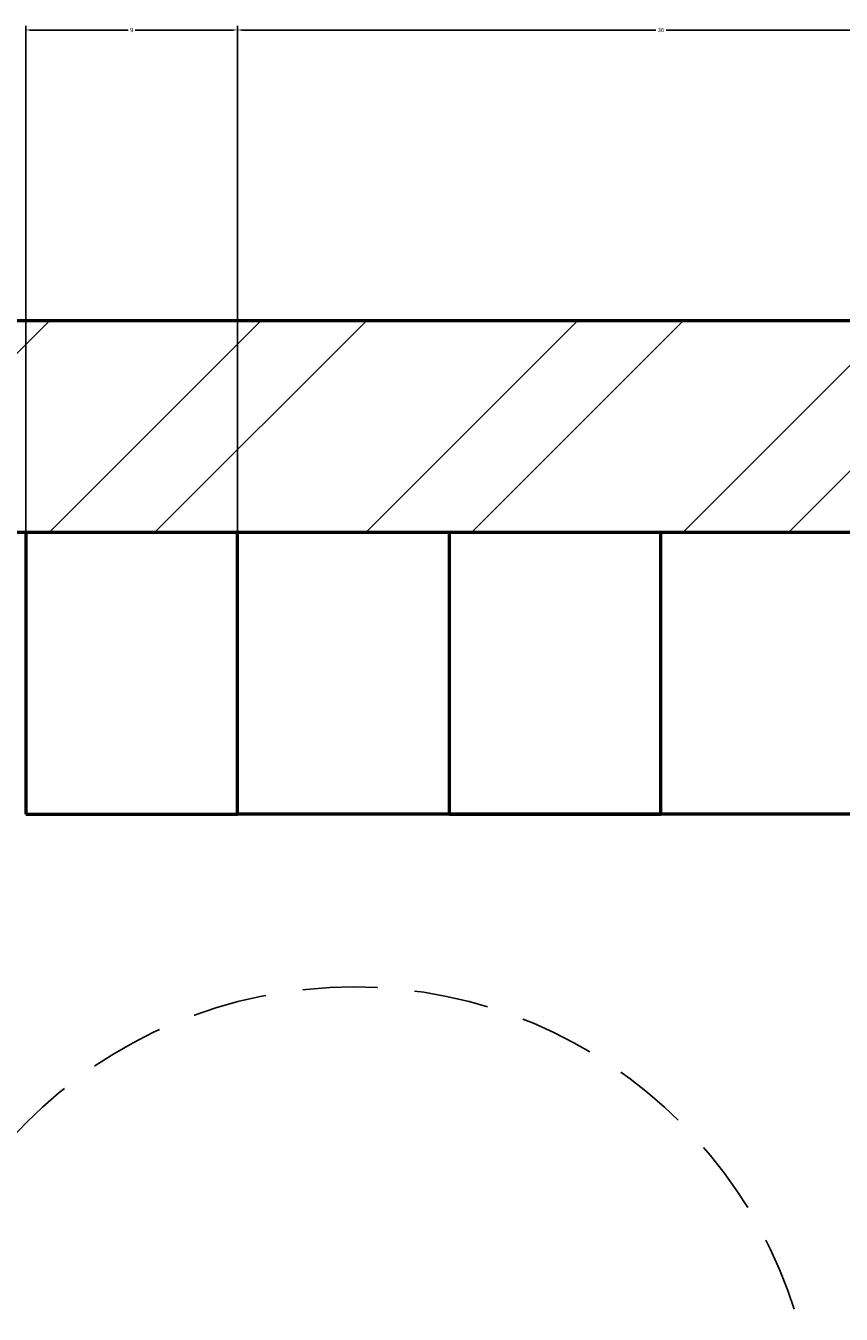
# Model space of a CAD drawing. Units: inches. Extents: x 2812 to 3051, y 1398 to 1659.
# Tile 64 of 65: x 2970 to 3005, y 1605 to 1659. Entities that reach past the tile are written whole.
import ezdxf

# ---------------------------------------------------------------- set-up
doc = ezdxf.new("R2010")
doc.units = ezdxf.units.IN
doc.linetypes.add('HIDDEN2', pattern=[4.7625, 3.175, -1.5875])
for name, color, linetype, lineweight in [('A-ANNO-DIMS', 2, 'Continuous', 18), ('S-CONC', 7, 'Continuous', 50), ('S-CONC-HIDN', 8, 'HIDDEN2', 25), ('S-CONC-PATT', 8, 'Continuous', 18)]:
    doc.layers.add(name, color=color, linetype=linetype, lineweight=lineweight)
doc.styles.get("Standard").update_dxf_attribs({"font": 'arial.ttf'})
doc.dimstyles.get("Standard").update_dxf_attribs({"dimtxt": 0.18, "dimasz": 0.18, "dimexe": 0.18, "dimexo": 0.0625, "dimgap": 0.09, "dimtad": 0, "dimtih": 1, "dimtoh": 1, "dimdec": 4, "dimzin": 0, "dimdsep": 46, "dimtxsty": 'Standard', "dimcen": 0.09, "dimadec": 0, "dimazin": 0, "dimtfac": 1, "dimtdec": 4, "dimtofl": 0, "dimtmove": 0, "dimatfit": 3, "dimfxl": 1, "dimtolj": 1, "dimtzin": 0, "dimarcsym": 0})

# ---------------------------------------------------------------- blocks, each defined once
blk = doc.blocks.new('*D23')
at = {"layer": 'A-ANNO-DIMS', "color": 0, "lineweight": -2, "transparency": 16777216}
for p, q in [((2970.385, 1625.882), (2970.385, 1659.35)), ((2970.565, 1659.17), (2974.736, 1659.17)), ((2979.205, 1659.17), (2975.034, 1659.17)), ((2979.385, 1625.882), (2979.385, 1659.35))]:
    blk.add_line(p, q, dxfattribs=at)
at = {"layer": 'A-ANNO-DIMS', "color": 0, "transparency": 16777216}
for points in [[(2970.565, 1659.2), (2970.565, 1659.14), (2970.385, 1659.17)], [(2979.205, 1659.2), (2979.205, 1659.14), (2979.385, 1659.17)]]:
    blk.add_solid(points, dxfattribs=at)
at = {"layer": 'Defpoints', "color": 0, "transparency": 16777216}
for p in [(2979.385, 1659.17), (2970.385, 1625.82), (2979.385, 1625.82)]:
    blk.add_point(p, dxfattribs=at)
at = {"layer": 'A-ANNO-DIMS', "color": 0, "transparency": 16777216, "insert": (2974.885, 1659.17), "char_height": 0.18, "attachment_point": 5}
blk.add_mtext('\\A1;9', dxfattribs=at)
blk = doc.blocks.new('*D24')
at = {"layer": 'A-ANNO-DIMS', "color": 0, "lineweight": -2, "transparency": 16777216}
for p, q in [((2979.385, 1625.882), (2979.385, 1659.35)), ((2979.565, 1659.17), (2997.166, 1659.17)), ((3015.205, 1659.17), (2997.604, 1659.17)), ((3015.385, 1625.882), (3015.385, 1659.35))]:
    blk.add_line(p, q, dxfattribs=at)
at = {"layer": 'A-ANNO-DIMS', "color": 0, "transparency": 16777216}
for points in [[(2979.565, 1659.2), (2979.565, 1659.14), (2979.385, 1659.17)], [(3015.205, 1659.2), (3015.205, 1659.14), (3015.385, 1659.17)]]:
    blk.add_solid(points, dxfattribs=at)
at = {"layer": 'Defpoints', "color": 0, "transparency": 16777216}
for p in [(3015.385, 1659.17), (2979.385, 1625.82), (3015.385, 1625.82)]:
    blk.add_point(p, dxfattribs=at)
at = {"layer": 'A-ANNO-DIMS', "color": 0, "transparency": 16777216, "insert": (2997.385, 1659.17), "char_height": 0.18, "attachment_point": 5}
blk.add_mtext('\\A1;36', dxfattribs=at)

msp = doc.modelspace()

# ---------------------------------------------------------------- hatches: boundary and pattern name
at = {"layer": 'S-CONC-PATT'}
h = msp.add_hatch(dxfattribs=at)
h.set_pattern_fill('ANSI32', color=256)
h.paths.add_polyline_path([(3027.3849, 1646.82), (2835.3849, 1646.82), (2835.3849, 1603.2296), (2844.3849, 1603.2296), (2844.3849, 1637.82), (3018.3849, 1637.82), (3018.3849, 1602.5441), (3027.3849, 1602.5441)])
h.paths.add_polyline_path([(2844.3849, 1594.2296), (2835.3849, 1594.2296), (2835.3849, 1550.82), (3027.3849, 1550.82), (3027.3849, 1593.5441), (3018.3849, 1593.5441), (3018.3849, 1559.82), (2844.3849, 1559.82)])
h.paths.add_polyline_path([(2844.3849, 1482.0354), (2835.3849, 1482.0354), (2835.3849, 1463.4959), (2844.3849, 1463.4959)])
h.paths.add_polyline_path([(2844.3849, 1461.4959), (2835.3849, 1461.4959), (2835.3849, 1416.0354), (2844.3849, 1416.0354)])
h.paths.add_polyline_path([(3027.3849, 1482.0354), (3018.3849, 1482.0354), (3018.3849, 1463.2854), (3027.3849, 1463.2854)])
h.paths.add_polyline_path([(3027.3849, 1461.2854), (3018.3849, 1461.2854), (3018.3849, 1416.0354), (3027.3849, 1416.0354)])
h.paths.add_polyline_path([(2961.3849, 1448.4738), (2952.3849, 1448.4738), (2952.3849, 1416.0354), (2961.3849, 1416.0354)])
h.paths.add_polyline_path([(2961.3849, 1462.3026), (2952.3849, 1462.3026), (2952.3849, 1450.4738), (2961.3849, 1450.4738)])
h.paths.add_polyline_path([(2961.3849, 1472.0354), (2952.3849, 1472.0354), (2952.3849, 1462.3026), (2961.3849, 1462.3026)])

# ---------------------------------------------------------------- linework, layer by layer
at = {"layer": 'S-CONC'}
for p, q in [((2835.3849, 1646.82), (3027.3849, 1646.82)), ((2844.3849, 1637.82), (3018.3849, 1637.82)), ((2970.3849, 1637.82), (2970.3849, 1625.82)), ((2979.3849, 1625.82), (2979.3849, 1637.82)), ((2979.3849, 1637.82), (2988.3849, 1637.82)), ((2988.3849, 1637.82), (2988.3849, 1625.82)), ((2997.3849, 1625.82), (2997.3849, 1637.82)), ((2997.3849, 1637.82), (3006.3849, 1637.82)), ((2970.3849, 1625.82), (2979.3849, 1625.82)), ((2997.3849, 1625.82), (2979.3849, 1625.82)), ((2988.3849, 1625.82), (2997.3849, 1625.82)), ((3015.3849, 1625.82), (2997.3849, 1625.82))]:
    msp.add_line(p, q, dxfattribs=at)
at = {"layer": 'S-CONC-HIDN'}
msp.add_circle((2984.3156, 1598.82), 19.6588, dxfattribs=at)

# ---------------------------------------------------------------- dimensions: what is measured, and where the dimension line sits
at = {"layer": 'A-ANNO-DIMS'}
for base, p1, p2, picture, middle in [((2979.3849, 1659.17), (2970.3849, 1625.82), (2979.3849, 1625.82), '*D23', (2974.8849, 1659.17)), ((3015.3849, 1659.17), (2979.3849, 1625.82), (3015.3849, 1625.82), '*D24', (2997.3849, 1659.17))]:
    dim = msp.add_linear_dim(base=base, p1=p1, p2=p2, dimstyle='Standard', override={"dimdec": 0, "dimlfac": 1, "dimrnd": 0, "dimzin": 0, "dimdsep": 46, "dimlunit": 2}, dxfattribs=at)
    dim.commit()
    dim.dimension.update_dxf_attribs({"geometry": picture, "text_midpoint": middle})

doc.saveas('drawing.dxf')
